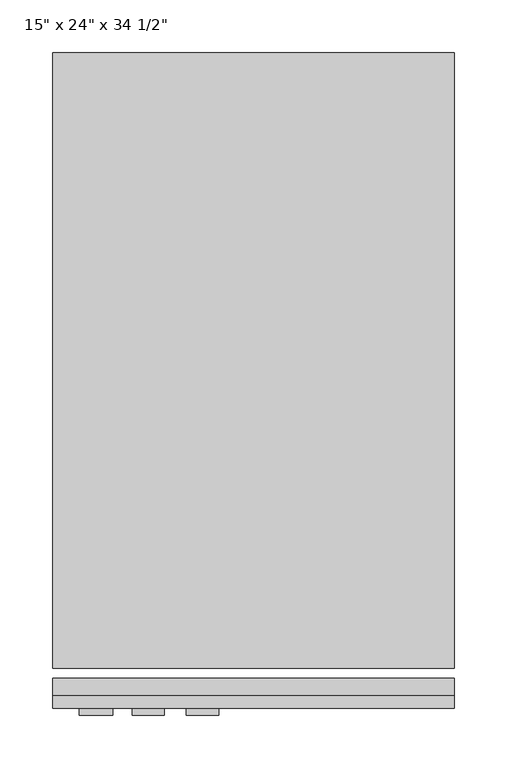
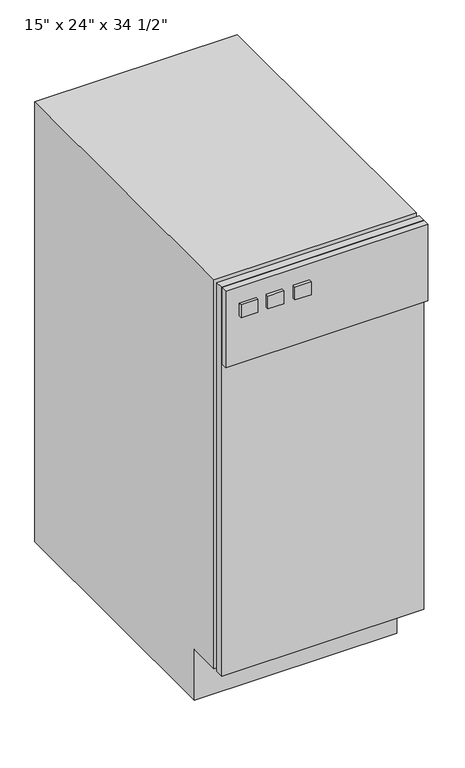
"""IFC4 building model written with IfcOpenShell, lengths in millimetres: proxy geometry."""

from ifc_helpers import new_model, si_unit, frame, origin, place, context, project, spatial, polyline, outline, extrude, source, transform, mapped, element, save


def proxy_db4bb64d(model_context):
    return source(origin(), model_context, "Body", "SweptSolid", [
        extrude(outline(polyline([(458.5174685, -38.3504352), (77.5174685, -38.3504352), (77.5174685, -22.4754352), (458.5174685, -22.4754352), (458.5174685, -38.3504352)])), frame((0.0, 0.0, 101.6), z_axis=(0.0, 0.0, 1.0), x_axis=(1.0, 0.0, 0.0)), (0.0, 0.0, 1.0), 774.7),
        extrude(outline(polyline([(458.5174685, -38.3504352), (458.5174685, -51.0504352), (77.5174685, -51.0504352), (77.5174685, -38.3504352), (458.5174685, -38.3504352)])), frame((0.0, 0.0, 723.9), z_axis=(0.0, 0.0, 1.0), x_axis=(1.0, 0.0, 0.0)), (0.0, 0.0, 1.0), 152.4),
        extrude(outline(polyline([(571.2495648, 0.0), (50.5495648, 0.0), (50.5495648, 101.6), (-12.9504352, 101.6), (-12.9504352, 876.3), (571.2495648, 876.3), (571.2495648, 0.0)])), frame((77.5174685, 0.0, 0.0), z_axis=(1.0, 0.0, 0.0), x_axis=(0.0, 1.0, 0.0)), (0.0, 0.0, 1.0), 381.0),
        extrude(outline(polyline([(134.6674685, -57.4004352), (102.9174685, -57.4004352), (102.9174685, -51.0504352), (134.6674685, -51.0504352), (134.6674685, -57.4004352)])), frame((0.0, 0.0, 818.6415009), z_axis=(0.0, 0.0, 1.0), x_axis=(1.0, 0.0, 0.0)), (0.0, 0.0, 1.0), 25.4),
        extrude(outline(polyline([(183.5847918, -57.4004352), (153.2389562, -57.4004352), (153.2389562, -51.0504352), (183.5847918, -51.0504352), (183.5847918, -57.4004352)])), frame((0.0, 0.0, 818.6415009), z_axis=(0.0, 0.0, 1.0), x_axis=(1.0, 0.0, 0.0)), (0.0, 0.0, 1.0), 25.4),
        extrude(outline(polyline([(234.869254, -57.4004352), (204.2199601, -57.4004352), (204.2199601, -51.0504352), (234.869254, -51.0504352), (234.869254, -57.4004352)])), frame((0.0, 0.0, 818.6415009), z_axis=(0.0, 0.0, 1.0), x_axis=(1.0, 0.0, 0.0)), (0.0, 0.0, 1.0), 25.4),
    ])


if __name__ == "__main__":
    model = new_model("IFC4")
    model_context = context("Model", 3, world=origin())
    ifc_project = project(units=[si_unit("LENGTHUNIT", "METRE", prefix="MILLI")], contexts=[model_context])
    site = spatial("IfcSite", under=ifc_project)
    building = spatial("IfcBuilding", under=site)
    placement = place(None, origin())
    proxy_shape = proxy_db4bb64d(model_context)
    element("IfcBuildingElementProxy", 1, Name="15\" x 24\" x 34 1/2\"", ObjectType="15\" x 24\" x 34 1/2\"", at=placement, inside=building, context=model_context, shape_type="MappedRepresentation", body=[
        mapped(proxy_shape, transform((0.0, 0.0, 0.0), x_axis=(1.0, 0.0, 0.0), y_axis=(0.0, 1.0, 0.0), z_axis=(0.0, 0.0, 1.0))),
    ])
    save(model, "model.ifc")

# Revit data of these elements
# Type "15\" x 24\" x 34 1/2\""
#   Label = "T"
#   Assembly Code = "E1090400"
#   Depth = 2' - 0"
#   Height = 2' - 10 1/2"
#   Width = 1' - 3"
#   Panel Face Material = Plastic, Opaque Black
#   Trach Compact. Material = Steel, Paint Finish, Ivory, Matte
#   Default Elevation = 0
# Element 1 (IfcBuildingElementProxy, "15\" x 24\" x 34 1/2\"")
#   Materials on its faces: "Steel, Paint Finish, Ivory, Matte", "Plastic, Opaque Black"
# Materials
#   "Plastic, Opaque Black": class "Plastic", colour RGB 0 0 0, transparency 0.7, Description = "Plastic, generic, opaque black", Cost = 0
#   "Steel, Paint Finish, Ivory, Matte": class "Metal", colour RGB 247 247 239, transparency 0, Description = "Steel, paint finish, ivory, matte", Cost = 0
